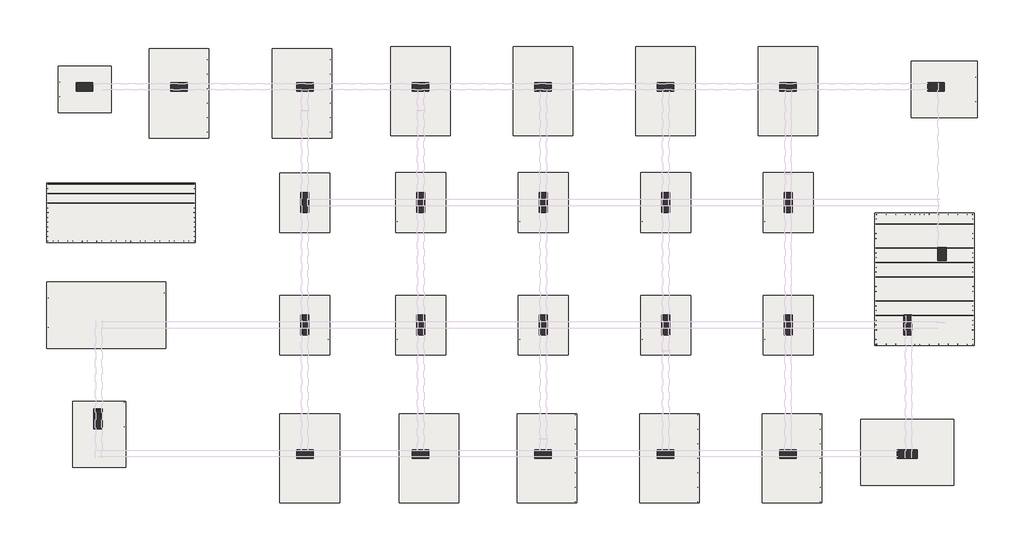
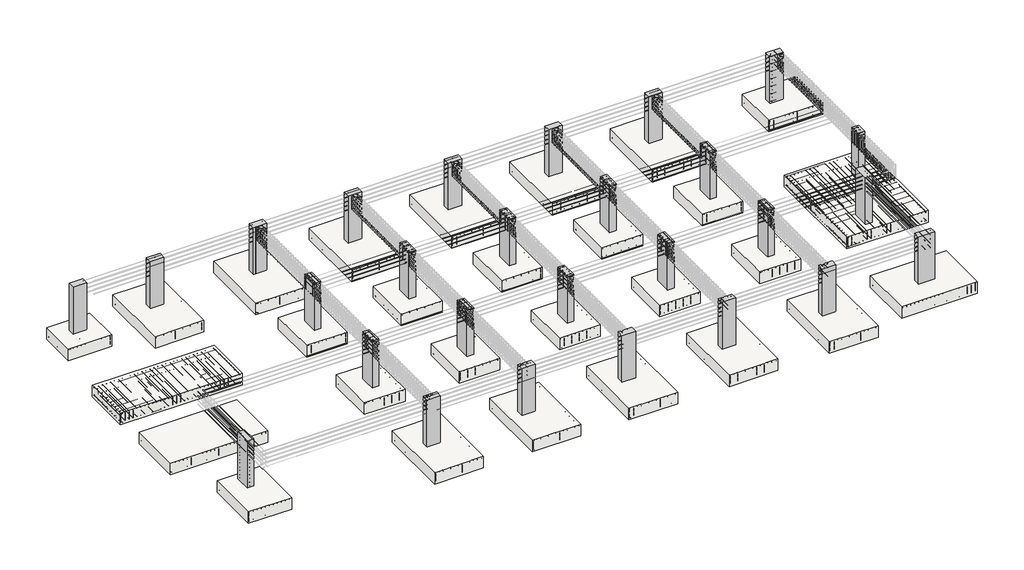
# One storey, part 1 of 16: 28 slabs, 27 columns.
"""IFC4 building model written with IfcOpenShell, lengths in millimetres."""

from ifc_helpers import new_model, si_unit, frame, origin, place, context, project, spatial, polyline, outline, extrude, faceted_brep, transform, mapped, element, save
from components import footing_rectangular_1400x1600x450_119851bf, footing_rectangular_1500x1800x450_b566de6d, footing_rectangular_1600x2000x450_9a9f7728, footing_rectangular_1800x2700x450_79bb3453, footing_rectangular_2000x1700x450_8886efa8, footing_rectangular_2800x2000x450_516ac05f, footing_rectangular_3000x4000x450_ea1acd88, footing_rectangular_3600x2000x450_36af6fae, footing_rectangular_4498x1800x450_c2833046

model = new_model("IFC4")

# Units and contexts
model_context = context("Model", 3, world=origin())
ifc_project = project(units=[si_unit("LENGTHUNIT", "METRE", prefix="MILLI")], contexts=[model_context])

# Site, building, storey
site = spatial("IfcSite", under=ifc_project)
building = spatial("IfcBuilding", under=site)
storey = spatial("IfcBuildingStorey", under=building, Elevation=-1828.8)

# Columns
placement = place(None, origin())
element("IfcColumn", 1, ObjectType="Concrete-Rectangular-Column : 250X400", at=placement, inside=storey, context=model_context, shape_type="SweptSolid", body=[
    extrude(outline(polyline([(10438.1883401, -29.1308992), (10438.1883401, -429.1308992), (10188.1883401, -429.1308992), (10188.1883401, -29.1308992), (10438.1883401, -29.1308992)])), frame((0.0, 0.0, -1828.8), z_axis=(0.0, 0.0, 1.0), x_axis=(1.0, 0.0, 0.0)), (0.0, 0.0, 1.0), 1828.8),
])
element("IfcColumn", 2, ObjectType="Concrete-Rectangular-Column : 250X500", at=placement, inside=storey, context=model_context, shape_type="SweptSolid", body=[
    extrude(outline(polyline([(-15828.3116599, 4945.8691009), (-15328.3116599, 4945.8691009), (-15328.3116599, 4695.8691009), (-15828.3116599, 4695.8691009), (-15828.3116599, 4945.8691009)])), frame((0.0, 0.0, -1828.8), z_axis=(0.0, 0.0, 1.0), x_axis=(1.0, 0.0, 0.0)), (0.0, 0.0, 1.0), 1828.8),
])
element("IfcColumn", 3, ObjectType="Concrete-Rectangular-Column : 250X500", at=placement, inside=storey, context=model_context, shape_type="SweptSolid", body=[
    extrude(outline(polyline([(-12978.3116599, 4945.8691009), (-12478.3116599, 4945.8691009), (-12478.3116599, 4695.8691009), (-12978.3116599, 4695.8691009), (-12978.3116599, 4945.8691009)])), frame((0.0, 0.0, -1828.8), z_axis=(0.0, 0.0, 1.0), x_axis=(1.0, 0.0, 0.0)), (0.0, 0.0, 1.0), 1828.8),
])
element("IfcColumn", 4, ObjectType="Concrete-Rectangular-Column : 250X500", at=placement, inside=storey, context=model_context, shape_type="SweptSolid", body=[
    extrude(outline(polyline([(-9178.2725801, 4945.8691009), (-8678.2725801, 4945.8691009), (-8678.2725801, 4695.8691009), (-9178.2725801, 4695.8691009), (-9178.2725801, 4945.8691009)])), frame((0.0, 0.0, -1828.8), z_axis=(0.0, 0.0, 1.0), x_axis=(1.0, 0.0, 0.0)), (0.0, 0.0, 1.0), 1828.8),
])
element("IfcColumn", 5, ObjectType="Concrete-Rectangular-Column : 250X500", at=placement, inside=storey, context=model_context, shape_type="SweptSolid", body=[
    extrude(outline(polyline([(-5678.2725801, 4945.8691009), (-5178.2725801, 4945.8691009), (-5178.2725801, 4695.8691009), (-5678.2725801, 4695.8691009), (-5678.2725801, 4945.8691009)])), frame((0.0, 0.0, -1828.8), z_axis=(0.0, 0.0, 1.0), x_axis=(1.0, 0.0, 0.0)), (0.0, 0.0, 1.0), 1828.8),
])
element("IfcColumn", 6, ObjectType="Concrete-Rectangular-Column : 250X500", at=placement, inside=storey, context=model_context, shape_type="SweptSolid", body=[
    extrude(outline(polyline([(-1978.2725801, 4945.8691009), (-1478.2725801, 4945.8691009), (-1478.2725801, 4695.8691009), (-1978.2725801, 4695.8691009), (-1978.2725801, 4945.8691009)])), frame((0.0, 0.0, -1828.8), z_axis=(0.0, 0.0, 1.0), x_axis=(1.0, 0.0, 0.0)), (0.0, 0.0, 1.0), 1828.8),
])
element("IfcColumn", 7, ObjectType="Concrete-Rectangular-Column : 250X500", at=placement, inside=storey, context=model_context, shape_type="SweptSolid", body=[
    extrude(outline(polyline([(1721.7274199, 4945.8691009), (2221.7274199, 4945.8691009), (2221.7274199, 4695.8691009), (1721.7274199, 4695.8691009), (1721.7274199, 4945.8691009)])), frame((0.0, 0.0, -1828.8), z_axis=(0.0, 0.0, 1.0), x_axis=(1.0, 0.0, 0.0)), (0.0, 0.0, 1.0), 1828.8),
])
element("IfcColumn", 8, ObjectType="Concrete-Rectangular-Column : 250X500", at=placement, inside=storey, context=model_context, shape_type="SweptSolid", body=[
    extrude(outline(polyline([(5421.7274199, 4945.8691009), (5921.7274199, 4945.8691009), (5921.7274199, 4695.8691009), (5421.7274199, 4695.8691009), (5421.7274199, 4945.8691009)])), frame((0.0, 0.0, -1828.8), z_axis=(0.0, 0.0, 1.0), x_axis=(1.0, 0.0, 0.0)), (0.0, 0.0, 1.0), 1828.8),
])
element("IfcColumn", 9, ObjectType="Concrete-Rectangular-Column : 250X500", at=placement, inside=storey, context=model_context, shape_type="Brep", body=[
    faceted_brep([(9888.1883401, 4942.7630349, 0.0), (9888.1883401, 4692.7630349, 0.0), (10388.1883401, 4692.7630349, 0.0), (10388.1883401, 4942.7630349, 0.0), (9888.1883401, 4942.7630349, -1828.8), (10388.1883401, 4942.7630349, -1828.8), (10388.1883401, 4692.7630349, -1828.8), (9888.1883401, 4692.7630349, -1828.8), (9888.1883401, 4942.7630349, -152.4), (9888.1883401, 4942.7630349, -600.0), (9888.1883401, 4692.7630349, -600.0), (9888.1883401, 4692.7630349, -152.4), (10388.1883401, 4692.7630349, -600.0), (10388.1883401, 4692.7630349, -152.4), (10388.1883401, 4942.7630349, -600.0), (10388.1883401, 4942.7630349, -152.4)], [[[0, 1, 2, 3]], [[4, 5, 6, 7]], [[1, 0, 8, 9, 4, 7, 10, 11]], [[2, 1, 11, 10, 7, 6, 12, 13]], [[3, 2, 13, 12, 6, 5, 14, 15]], [[0, 3, 15, 14, 5, 4, 9, 8]]]),
])
element("IfcColumn", 10, ObjectType="Concrete-Rectangular-Column : 250X500", at=placement, inside=storey, context=model_context, shape_type="SweptSolid", body=[
    extrude(outline(polyline([(5421.7274199, -6154.1308991), (5921.7274199, -6154.1308991), (5921.7274199, -6404.1308991), (5421.7274199, -6404.1308991), (5421.7274199, -6154.1308991)])), frame((0.0, 0.0, -1828.8), z_axis=(0.0, 0.0, 1.0), x_axis=(1.0, 0.0, 0.0)), (0.0, 0.0, 1.0), 1828.8),
])
element("IfcColumn", 11, ObjectType="Concrete-Rectangular-Column : 250X500", at=placement, inside=storey, context=model_context, shape_type="SweptSolid", body=[
    extrude(outline(polyline([(1721.7274199, -6154.1308991), (2221.7274199, -6154.1308991), (2221.7274199, -6404.1308991), (1721.7274199, -6404.1308991), (1721.7274199, -6154.1308991)])), frame((0.0, 0.0, -1828.8), z_axis=(0.0, 0.0, 1.0), x_axis=(1.0, 0.0, 0.0)), (0.0, 0.0, 1.0), 1828.8),
])
element("IfcColumn", 12, ObjectType="Concrete-Rectangular-Column : 250X500", at=placement, inside=storey, context=model_context, shape_type="SweptSolid", body=[
    extrude(outline(polyline([(-1978.2725801, -6154.1308991), (-1478.2725801, -6154.1308991), (-1478.2725801, -6404.1308991), (-1978.2725801, -6404.1308991), (-1978.2725801, -6154.1308991)])), frame((0.0, 0.0, -1828.8), z_axis=(0.0, 0.0, 1.0), x_axis=(1.0, 0.0, 0.0)), (0.0, 0.0, 1.0), 1828.8),
])
element("IfcColumn", 13, ObjectType="Concrete-Rectangular-Column : 250X500", at=placement, inside=storey, context=model_context, shape_type="SweptSolid", body=[
    extrude(outline(polyline([(-5678.2725801, -6154.1308991), (-5178.2725801, -6154.1308991), (-5178.2725801, -6404.1308991), (-5678.2725801, -6404.1308991), (-5678.2725801, -6154.1308991)])), frame((0.0, 0.0, -1828.8), z_axis=(0.0, 0.0, 1.0), x_axis=(1.0, 0.0, 0.0)), (0.0, 0.0, 1.0), 1828.8),
])
element("IfcColumn", 14, ObjectType="Concrete-Rectangular-Column : 250X500", at=placement, inside=storey, context=model_context, shape_type="SweptSolid", body=[
    extrude(outline(polyline([(-9178.2725801, -6154.1308991), (-8678.2725801, -6154.1308991), (-8678.2725801, -6404.1308991), (-9178.2725801, -6404.1308991), (-9178.2725801, -6154.1308991)])), frame((0.0, 0.0, -1828.8), z_axis=(0.0, 0.0, 1.0), x_axis=(1.0, 0.0, 0.0)), (0.0, 0.0, 1.0), 1828.8),
])
element("IfcColumn", 15, ObjectType="Concrete-Rectangular-Column : 250X600", at=placement, inside=storey, context=model_context, shape_type="SweptSolid", body=[
    extrude(outline(polyline([(-8803.2725801, 1620.8691009), (-8803.2725801, 1020.8691009), (-9053.2725801, 1020.8691009), (-9053.2725801, 1620.8691009), (-8803.2725801, 1620.8691009)])), frame((0.0, 0.0, -1828.8), z_axis=(0.0, 0.0, 1.0), x_axis=(1.0, 0.0, 0.0)), (0.0, 0.0, 1.0), 1828.8),
])
element("IfcColumn", 16, ObjectType="Concrete-Rectangular-Column : 250X600", at=placement, inside=storey, context=model_context, shape_type="SweptSolid", body=[
    extrude(outline(polyline([(-5303.2725801, 1622.3111779), (-5303.2725801, 1022.3111779), (-5553.2725801, 1022.3111779), (-5553.2725801, 1622.3111779), (-5303.2725801, 1622.3111779)])), frame((0.0, 0.0, -1828.8), z_axis=(0.0, 0.0, 1.0), x_axis=(1.0, 0.0, 0.0)), (0.0, 0.0, 1.0), 1828.8),
])
element("IfcColumn", 17, ObjectType="Concrete-Rectangular-Column : 250X600", at=placement, inside=storey, context=model_context, shape_type="SweptSolid", body=[
    extrude(outline(polyline([(-1603.2725801, 1622.3111779), (-1603.2725801, 1022.3111779), (-1853.2725801, 1022.3111779), (-1853.2725801, 1622.3111779), (-1603.2725801, 1622.3111779)])), frame((0.0, 0.0, -1828.8), z_axis=(0.0, 0.0, 1.0), x_axis=(1.0, 0.0, 0.0)), (0.0, 0.0, 1.0), 1828.8),
])
element("IfcColumn", 18, ObjectType="Concrete-Rectangular-Column : 250X600", at=placement, inside=storey, context=model_context, shape_type="SweptSolid", body=[
    extrude(outline(polyline([(2096.7274199, 1622.3111779), (2096.7274199, 1022.3111779), (1846.7274199, 1022.3111779), (1846.7274199, 1622.3111779), (2096.7274199, 1622.3111779)])), frame((0.0, 0.0, -1828.8), z_axis=(0.0, 0.0, 1.0), x_axis=(1.0, 0.0, 0.0)), (0.0, 0.0, 1.0), 1828.8),
])
element("IfcColumn", 19, ObjectType="Concrete-Rectangular-Column : 250X600", at=placement, inside=storey, context=model_context, shape_type="SweptSolid", body=[
    extrude(outline(polyline([(5796.7274199, 1622.3111779), (5796.7274199, 1022.3111779), (5546.7274199, 1022.3111779), (5546.7274199, 1622.3111779), (5796.7274199, 1622.3111779)])), frame((0.0, 0.0, -1828.8), z_axis=(0.0, 0.0, 1.0), x_axis=(1.0, 0.0, 0.0)), (0.0, 0.0, 1.0), 1828.8),
])
element("IfcColumn", 20, ObjectType="Concrete-Rectangular-Column : 250X600", at=placement, inside=storey, context=model_context, shape_type="SweptSolid", body=[
    extrude(outline(polyline([(9406.9733834, -2079.1308991), (9406.9733834, -2679.1308991), (9156.9733834, -2679.1308991), (9156.9733834, -2079.1308991), (9406.9733834, -2079.1308991)])), frame((0.0, 0.0, -1828.8), z_axis=(0.0, 0.0, 1.0), x_axis=(1.0, 0.0, 0.0)), (0.0, 0.0, 1.0), 1828.8),
])
element("IfcColumn", 21, ObjectType="Concrete-Rectangular-Column : 250X600", at=placement, inside=storey, context=model_context, shape_type="SweptSolid", body=[
    extrude(outline(polyline([(5796.7274199, -2079.1308991), (5796.7274199, -2679.1308991), (5546.7274199, -2679.1308991), (5546.7274199, -2079.1308991), (5796.7274199, -2079.1308991)])), frame((0.0, 0.0, -1828.8), z_axis=(0.0, 0.0, 1.0), x_axis=(1.0, 0.0, 0.0)), (0.0, 0.0, 1.0), 1828.8),
])
element("IfcColumn", 22, ObjectType="Concrete-Rectangular-Column : 250X600", at=placement, inside=storey, context=model_context, shape_type="SweptSolid", body=[
    extrude(outline(polyline([(2096.7274199, -2079.1308991), (2096.7274199, -2679.1308991), (1846.7274199, -2679.1308991), (1846.7274199, -2079.1308991), (2096.7274199, -2079.1308991)])), frame((0.0, 0.0, -1828.8), z_axis=(0.0, 0.0, 1.0), x_axis=(1.0, 0.0, 0.0)), (0.0, 0.0, 1.0), 1828.8),
])
element("IfcColumn", 23, ObjectType="Concrete-Rectangular-Column : 250X600", at=placement, inside=storey, context=model_context, shape_type="Brep", body=[
    faceted_brep([(-1603.2725801, -2079.1308991, 0.0), (-1853.2725801, -2079.1308991, 0.0), (-1853.2725801, -2679.1308991, 0.0), (-1603.2725801, -2679.1308991, 0.0), (-1603.2725801, -2079.1308991, -1828.8), (-1603.2725801, -2679.1308991, -1828.8), (-1853.2725801, -2679.1308991, -1828.8), (-1853.2725801, -2079.1308991, -1828.8), (-1603.2725801, -2079.1308991, -152.4), (-1603.2725801, -2079.1308991, -600.0), (-1853.2725801, -2079.1308991, -600.0), (-1853.2725801, -2079.1308991, -152.4)], [[[0, 1, 2, 3]], [[4, 5, 6, 7]], [[1, 0, 8, 9, 4, 7, 10, 11]], [[2, 1, 11, 10, 7, 6]], [[3, 2, 6, 5]], [[0, 3, 5, 4, 9, 8]]]),
])
element("IfcColumn", 24, ObjectType="Concrete-Rectangular-Column : 250X600", at=placement, inside=storey, context=model_context, shape_type="SweptSolid", body=[
    extrude(outline(polyline([(-5303.2725801, -2079.1308991), (-5303.2725801, -2679.1308991), (-5553.2725801, -2679.1308991), (-5553.2725801, -2079.1308991), (-5303.2725801, -2079.1308991)])), frame((0.0, 0.0, -1828.8), z_axis=(0.0, 0.0, 1.0), x_axis=(1.0, 0.0, 0.0)), (0.0, 0.0, 1.0), 1828.8),
])
element("IfcColumn", 25, ObjectType="Concrete-Rectangular-Column : 250X600", at=placement, inside=storey, context=model_context, shape_type="Brep", body=[
    faceted_brep([(-8803.2725801, -2079.1308991, 0.0), (-9053.2725801, -2079.1308991, 0.0), (-9053.2725801, -2679.1308991, 0.0), (-8803.2725801, -2679.1308991, 0.0), (-8803.2725801, -2079.1308991, -1828.8), (-8803.2725801, -2679.1308991, -1828.8), (-9053.2725801, -2679.1308991, -1828.8), (-9053.2725801, -2079.1308991, -1828.8), (-8803.2725801, -2079.1308991, -152.4), (-8803.2725801, -2079.1308991, -600.0), (-9053.2725801, -2079.1308991, -600.0), (-9053.2725801, -2079.1308991, -152.4)], [[[0, 1, 2, 3]], [[4, 5, 6, 7]], [[1, 0, 8, 9, 4, 7, 10, 11]], [[2, 1, 11, 10, 7, 6]], [[3, 2, 6, 5]], [[0, 3, 5, 4, 9, 8]]]),
])
element("IfcColumn", 26, ObjectType="Concrete-Rectangular-Column : 250X600", at=placement, inside=storey, context=model_context, shape_type="SweptSolid", body=[
    extrude(outline(polyline([(-15050.5528212, -4909.1308991), (-15050.5528212, -5509.1308991), (-15300.5528212, -5509.1308991), (-15300.5528212, -4909.1308991), (-15050.5528212, -4909.1308991)])), frame((0.0, 0.0, -1828.8), z_axis=(0.0, 0.0, 1.0), x_axis=(1.0, 0.0, 0.0)), (0.0, 0.0, 1.0), 1828.8),
])
element("IfcColumn", 27, ObjectType="Concrete-Rectangular-Column : 250X600", at=placement, inside=storey, context=model_context, shape_type="Brep", body=[
    faceted_brep([(8968.1883401, -6153.1308991, 0.0), (8968.1883401, -6403.1308991, 0.0), (9568.1883401, -6403.1308991, 0.0), (9568.1883401, -6153.1308991, 0.0), (8968.1883401, -6153.1308991, -1828.8), (9568.1883401, -6153.1308991, -1828.8), (9568.1883401, -6403.1308991, -1828.8), (8968.1883401, -6403.1308991, -1828.8), (8968.1883401, -6153.1308991, -152.4), (8968.1883401, -6153.1308991, -600.0), (8968.1883401, -6403.1308991, -600.0), (8968.1883401, -6403.1308991, -152.4)], [[[0, 1, 2, 3]], [[4, 5, 6, 7]], [[1, 0, 8, 9, 4, 7, 10, 11]], [[2, 1, 11, 10, 7, 6]], [[3, 2, 6, 5]], [[0, 3, 5, 4, 9, 8]]]),
])

# Slabs
footing_rectangular_1400x1600x450_shape = footing_rectangular_1400x1600x450_119851bf(model_context)
element("IfcSlab", 28, ObjectType="Footing-Rectangular : 1400X1600X450", at=placement, inside=storey, context=model_context, shape_type="MappedRepresentation", body=[
    mapped(footing_rectangular_1400x1600x450_shape, transform((-15578.3116599, 4745.8691009, -1828.8), x_axis=(0.0, 1.0, 0.0), y_axis=(-1.0, 0.0, 0.0), z_axis=(0.0, 0.0, 1.0))),
])
footing_rectangular_1500x1800x450_shape = footing_rectangular_1500x1800x450_b566de6d(model_context)
element("IfcSlab", 29, ObjectType="Footing-Rectangular : 1500X1800X450", at=placement, inside=storey, context=model_context, shape_type="MappedRepresentation", body=[
    mapped(footing_rectangular_1500x1800x450_shape, transform((-8929.3240997, 1322.3111779, -1828.8), x_axis=(0.0, 1.0, 0.0), y_axis=(-1.0, 0.0, 0.0), z_axis=(0.0, 0.0, 1.0))),
])
element("IfcSlab", 30, ObjectType="Footing-Rectangular : 1500X1800X450", at=placement, inside=storey, context=model_context, shape_type="MappedRepresentation", body=[
    mapped(footing_rectangular_1500x1800x450_shape, transform((-5428.2725801, 1323.7532549, -1828.8), x_axis=(0.0, 1.0, 0.0), y_axis=(-1.0, 0.0, 0.0), z_axis=(0.0, 0.0, 1.0))),
])
element("IfcSlab", 31, ObjectType="Footing-Rectangular : 1500X1800X450", at=placement, inside=storey, context=model_context, shape_type="MappedRepresentation", body=[
    mapped(footing_rectangular_1500x1800x450_shape, transform((-1728.2725801, 1323.7532549, -1828.8), x_axis=(0.0, 1.0, 0.0), y_axis=(-1.0, 0.0, 0.0), z_axis=(0.0, 0.0, 1.0))),
])
element("IfcSlab", 32, ObjectType="Footing-Rectangular : 1500X1800X450", at=placement, inside=storey, context=model_context, shape_type="MappedRepresentation", body=[
    mapped(footing_rectangular_1500x1800x450_shape, transform((1971.7274199, 1323.7532549, -1828.8), x_axis=(0.0, 1.0, 0.0), y_axis=(-1.0, 0.0, 0.0), z_axis=(0.0, 0.0, 1.0))),
])
element("IfcSlab", 33, ObjectType="Footing-Rectangular : 1500X1800X450", at=placement, inside=storey, context=model_context, shape_type="MappedRepresentation", body=[
    mapped(footing_rectangular_1500x1800x450_shape, transform((5671.7274199, 1323.7532549, -1828.8), x_axis=(0.0, 1.0, 0.0), y_axis=(-1.0, 0.0, 0.0), z_axis=(0.0, 0.0, 1.0))),
])
element("IfcSlab", 34, ObjectType="Footing-Rectangular : 1500X1800X450", at=placement, inside=storey, context=model_context, shape_type="MappedRepresentation", body=[
    mapped(footing_rectangular_1500x1800x450_shape, transform((5671.7274199, -2377.6888221, -1828.8), x_axis=(0.0, 1.0, 0.0), y_axis=(-1.0, 0.0, 0.0), z_axis=(0.0, 0.0, 1.0))),
])
element("IfcSlab", 35, ObjectType="Footing-Rectangular : 1500X1800X450", at=placement, inside=storey, context=model_context, shape_type="MappedRepresentation", body=[
    mapped(footing_rectangular_1500x1800x450_shape, transform((1971.7274199, -2377.6888221, -1828.8), x_axis=(0.0, 1.0, 0.0), y_axis=(-1.0, 0.0, 0.0), z_axis=(0.0, 0.0, 1.0))),
])
element("IfcSlab", 36, ObjectType="Footing-Rectangular : 1500X1800X450", at=placement, inside=storey, context=model_context, shape_type="MappedRepresentation", body=[
    mapped(footing_rectangular_1500x1800x450_shape, transform((-1728.2725801, -2377.6888221, -1828.8), x_axis=(0.0, 1.0, 0.0), y_axis=(-1.0, 0.0, 0.0), z_axis=(0.0, 0.0, 1.0))),
])
element("IfcSlab", 37, ObjectType="Footing-Rectangular : 1500X1800X450", at=placement, inside=storey, context=model_context, shape_type="MappedRepresentation", body=[
    mapped(footing_rectangular_1500x1800x450_shape, transform((-5428.2725801, -2377.6888221, -1828.8), x_axis=(0.0, 1.0, 0.0), y_axis=(-1.0, 0.0, 0.0), z_axis=(0.0, 0.0, 1.0))),
])
element("IfcSlab", 38, ObjectType="Footing-Rectangular : 1500X1800X450", at=placement, inside=storey, context=model_context, shape_type="MappedRepresentation", body=[
    mapped(footing_rectangular_1500x1800x450_shape, transform((-8928.2725801, -2377.6888221, -1828.8), x_axis=(0.0, 1.0, 0.0), y_axis=(-1.0, 0.0, 0.0), z_axis=(0.0, 0.0, 1.0))),
])
footing_rectangular_1600x2000x450_shape = footing_rectangular_1600x2000x450_9a9f7728(model_context)
element("IfcSlab", 39, ObjectType="Footing-Rectangular : 1600X2000X450", at=placement, inside=storey, context=model_context, shape_type="MappedRepresentation", body=[
    mapped(footing_rectangular_1600x2000x450_shape, transform((-15130.5528212, -5679.1308991, -1828.8), x_axis=(0.0, 1.0, 0.0), y_axis=(-1.0, 0.0, 0.0), z_axis=(0.0, 0.0, 1.0))),
])
footing_rectangular_1800x2700x450_shape = footing_rectangular_1800x2700x450_79bb3453(model_context)
element("IfcSlab", 40, ObjectType="Footing-Rectangular : 1800X2700X450", at=placement, inside=storey, context=model_context, shape_type="MappedRepresentation", body=[
    mapped(footing_rectangular_1800x2700x450_shape, transform((-12724.5266165, 4620.8691009, -1828.8), x_axis=(0.0, 1.0, 0.0), y_axis=(-1.0, 0.0, 0.0), z_axis=(0.0, 0.0, 1.0))),
])
element("IfcSlab", 41, ObjectType="Footing-Rectangular : 1800X2700X450", at=placement, inside=storey, context=model_context, shape_type="MappedRepresentation", body=[
    mapped(footing_rectangular_1800x2700x450_shape, transform((-9008.0266166, 4620.8691009, -1828.8), x_axis=(0.0, 1.0, 0.0), y_axis=(-1.0, 0.0, 0.0), z_axis=(0.0, 0.0, 1.0))),
])
element("IfcSlab", 42, ObjectType="Footing-Rectangular : 1800X2700X450", at=placement, inside=storey, context=model_context, shape_type="MappedRepresentation", body=[
    mapped(footing_rectangular_1800x2700x450_shape, transform((-5433.0266166, 4692.7630349, -1828.8), x_axis=(0.0, 1.0, 0.0), y_axis=(-1.0, 0.0, 0.0), z_axis=(0.0, 0.0, 1.0))),
])
element("IfcSlab", 43, ObjectType="Footing-Rectangular : 1800X2700X450", at=placement, inside=storey, context=model_context, shape_type="MappedRepresentation", body=[
    mapped(footing_rectangular_1800x2700x450_shape, transform((-1733.0266166, 4692.7630349, -1828.8), x_axis=(0.0, 1.0, 0.0), y_axis=(-1.0, 0.0, 0.0), z_axis=(0.0, 0.0, 1.0))),
])
element("IfcSlab", 44, ObjectType="Footing-Rectangular : 1800X2700X450", at=placement, inside=storey, context=model_context, shape_type="MappedRepresentation", body=[
    mapped(footing_rectangular_1800x2700x450_shape, transform((1966.9733834, 4692.7630349, -1828.8), x_axis=(0.0, 1.0, 0.0), y_axis=(-1.0, 0.0, 0.0), z_axis=(0.0, 0.0, 1.0))),
])
element("IfcSlab", 45, ObjectType="Footing-Rectangular : 1800X2700X450", at=placement, inside=storey, context=model_context, shape_type="MappedRepresentation", body=[
    mapped(footing_rectangular_1800x2700x450_shape, transform((5666.9733834, 4692.7630349, -1828.8), x_axis=(0.0, 1.0, 0.0), y_axis=(-1.0, 0.0, 0.0), z_axis=(0.0, 0.0, 1.0))),
])
element("IfcSlab", 46, ObjectType="Footing-Rectangular : 1800X2700X450", at=placement, inside=storey, context=model_context, shape_type="MappedRepresentation", body=[
    mapped(footing_rectangular_1800x2700x450_shape, transform((5791.9733834, -6408.4085501, -1828.8), x_axis=(0.0, 1.0, 0.0), y_axis=(-1.0, 0.0, 0.0), z_axis=(0.0, 0.0, 1.0))),
])
element("IfcSlab", 47, ObjectType="Footing-Rectangular : 1800X2700X450", at=placement, inside=storey, context=model_context, shape_type="MappedRepresentation", body=[
    mapped(footing_rectangular_1800x2700x450_shape, transform((2091.9733834, -6408.4085501, -1828.8), x_axis=(0.0, 1.0, 0.0), y_axis=(-1.0, 0.0, 0.0), z_axis=(0.0, 0.0, 1.0))),
])
element("IfcSlab", 48, ObjectType="Footing-Rectangular : 1800X2700X450", at=placement, inside=storey, context=model_context, shape_type="MappedRepresentation", body=[
    mapped(footing_rectangular_1800x2700x450_shape, transform((-1608.0266166, -6408.4085501, -1828.8), x_axis=(0.0, 1.0, 0.0), y_axis=(-1.0, 0.0, 0.0), z_axis=(0.0, 0.0, 1.0))),
])
element("IfcSlab", 49, ObjectType="Footing-Rectangular : 1800X2700X450", at=placement, inside=storey, context=model_context, shape_type="MappedRepresentation", body=[
    mapped(footing_rectangular_1800x2700x450_shape, transform((-5178.2725801, -6408.4085501, -1828.8), x_axis=(0.0, 1.0, 0.0), y_axis=(-1.0, 0.0, 0.0), z_axis=(0.0, 0.0, 1.0))),
])
element("IfcSlab", 50, ObjectType="Footing-Rectangular : 1800X2700X450", at=placement, inside=storey, context=model_context, shape_type="MappedRepresentation", body=[
    mapped(footing_rectangular_1800x2700x450_shape, transform((-8778.2725801, -6408.4085501, -1828.8), x_axis=(0.0, 1.0, 0.0), y_axis=(-1.0, 0.0, 0.0), z_axis=(0.0, 0.0, 1.0))),
])
footing_rectangular_2000x1700x450_shape = footing_rectangular_2000x1700x450_8886efa8(model_context)
element("IfcSlab", 51, ObjectType="Footing-Rectangular : 2000X1700X450", at=placement, inside=storey, context=model_context, shape_type="MappedRepresentation", body=[
    mapped(footing_rectangular_2000x1700x450_shape, transform((10388.1883401, 4745.8691009, -1828.8), x_axis=(0.0, 1.0, 0.0), y_axis=(-1.0, 0.0, 0.0), z_axis=(0.0, 0.0, 1.0))),
])
footing_rectangular_2800x2000x450_shape = footing_rectangular_2800x2000x450_516ac05f(model_context)
element("IfcSlab", 52, ObjectType="Footing-Rectangular : 2800X2000X450", at=placement, inside=storey, context=model_context, shape_type="MappedRepresentation", body=[
    mapped(footing_rectangular_2800x2000x450_shape, transform((9268.1883401, -6228.1308991, -1828.8), x_axis=(0.0, 1.0, 0.0), y_axis=(-1.0, 0.0, 0.0), z_axis=(0.0, 0.0, 1.0))),
])
footing_rectangular_3000x4000x450_shape = footing_rectangular_3000x4000x450_ea1acd88(model_context)
element("IfcSlab", 53, ObjectType="Footing-Rectangular : 3000X4000X450", at=placement, inside=storey, context=model_context, shape_type="MappedRepresentation", body=[
    mapped(footing_rectangular_3000x4000x450_shape, transform((9788.1883401, -996.6308991, -1828.8), x_axis=(0.0, 1.0, 0.0), y_axis=(-1.0, 0.0, 0.0), z_axis=(0.0, 0.0, 1.0))),
])
footing_rectangular_3600x2000x450_shape = footing_rectangular_3600x2000x450_36af6fae(model_context)
element("IfcSlab", 54, ObjectType="Footing-Rectangular : 3600X2000X450", at=placement, inside=storey, context=model_context, shape_type="MappedRepresentation", body=[
    mapped(footing_rectangular_3600x2000x450_shape, transform((-14928.3116599, -2079.1308991, -1828.8), x_axis=(0.0, 1.0, 0.0), y_axis=(-1.0, 0.0, 0.0), z_axis=(0.0, 0.0, 1.0))),
])
footing_rectangular_4498x1800x450_shape = footing_rectangular_4498x1800x450_c2833046(model_context)
element("IfcSlab", 55, ObjectType="Footing-Rectangular : 4498X1800X450", at=placement, inside=storey, context=model_context, shape_type="MappedRepresentation", body=[
    mapped(footing_rectangular_4498x1800x450_shape, transform((-14479.278345, 1020.8691009, -1828.8), x_axis=(0.0, 1.0, 0.0), y_axis=(-1.0, 0.0, 0.0), z_axis=(0.0, 0.0, 1.0))),
])

save(model, "model.ifc")

# Revit data of these elements
# Type "Concrete-Rectangular-Column : 250X400"
#   b = 0' - 9.84252"
#   h = 1' - 3.74803"
#   Structural Material [instance default] = Concrete, Cast-in-Place gray
# Type "Concrete-Rectangular-Column : 250X500"
#   b = 0' - 9.84252"
#   h = 1' - 7.68504"
#   Structural Material [instance default] = Concrete, Cast-in-Place gray
# Type "Concrete-Rectangular-Column : 250X600"
#   b = 0' - 9.84252"
#   h = 1' - 11.62205"
#   Structural Material [instance default] = Concrete, Cast-in-Place gray
# Type "Footing-Rectangular : 1400X1600X450"
#   Width = 4' - 7.11811"
#   Length = 5' - 2.99213"
#   Foundation Thickness = 1' - 5.71654"
#   Structural Material [instance default] = Concrete - Cast-in-Place Concrete
#   Assembly Code = ""
# Type "Footing-Rectangular : 1500X1800X450"
#   Width = 5' - 10.86614"
#   Length = 4' - 11.05512"
#   Foundation Thickness = 1' - 5.71654"
#   Structural Material [instance default] = Concrete - Cast-in-Place Concrete
#   Assembly Code = ""
# Type "Footing-Rectangular : 1600X2000X450"
#   Width = 6' - 6.74016"
#   Length = 5' - 2.99213"
#   Foundation Thickness = 1' - 5.71654"
#   Structural Material [instance default] = Concrete - Cast-in-Place Concrete
#   Assembly Code = ""
# Type "Footing-Rectangular : 1800X2700X450"
#   Width = 8' - 10.29921"
#   Length = 5' - 10.86614"
#   Foundation Thickness = 1' - 5.71654"
#   Structural Material [instance default] = Concrete - Cast-in-Place Concrete
#   Assembly Code = ""
# Type "Footing-Rectangular : 2000X1700X450"
#   Width = 5' - 6.92913"
#   Length = 6' - 6.74016"
#   Foundation Thickness = 1' - 5.71654"
#   Structural Material [instance default] = Concrete - Cast-in-Place Concrete
#   Assembly Code = ""
# Type "Footing-Rectangular : 2800X2000X450"
#   Width = 6' - 6.74016"
#   Length = 9' - 2.23622"
#   Foundation Thickness = 1' - 5.71654"
#   Structural Material [instance default] = Concrete - Cast-in-Place Concrete
#   Assembly Code = ""
# Type "Footing-Rectangular : 3000X4000X450"
#   Width = 13' - 1.48031"
#   Length = 9' - 10.11024"
#   Foundation Thickness = 1' - 5.71654"
#   Structural Material [instance default] = Concrete - Cast-in-Place Concrete
#   Assembly Code = ""
# Type "Footing-Rectangular : 3600X2000X450"
#   Width = 6' - 6.74016"
#   Length = 11' - 9.73228"
#   Foundation Thickness = 1' - 5.71654"
#   Structural Material [instance default] = Concrete - Cast-in-Place Concrete
#   Assembly Code = ""
# Type "Footing-Rectangular : 4498X1800X450"
#   Width = 5' - 10.86614"
#   Length = 14' - 9.08661"
#   Foundation Thickness = 1' - 5.71654"
#   Structural Material [instance default] = Concrete - Cast-in-Place Concrete
#   Assembly Code = ""
# Element 1 (IfcColumn, "Concrete-Rectangular-Column : 250X400")
#   Structural Material = Concrete, Cast-in-Place gray
#   Phase Created = New Construction
#   Materials on its faces: "Concrete, Cast-in-Place gray"
# Elements 2, 3, 4, 5, 6, 7, 8, 9, 10, 11, 12, 13, 14 (IfcColumn, "Concrete-Rectangular-Column : 250X500")
#   Structural Material = Concrete, Cast-in-Place gray
#   Phase Created = New Construction
#   Materials on its faces: "Concrete, Cast-in-Place gray"
# Elements 15, 16, 17, 18, 19, 20, 21, 22, 23, 24, 25, 26, 27 (IfcColumn, "Concrete-Rectangular-Column : 250X600")
#   Structural Material = Concrete, Cast-in-Place gray
#   Phase Created = New Construction
#   Materials on its faces: "Concrete, Cast-in-Place gray"
# Element 28 (IfcSlab, "Footing-Rectangular : 1400X1600X450")
#   Structural Material = Concrete - Cast-in-Place Concrete
#   Phase Created = New Construction
#   Materials on its faces: "Concrete - Cast-in-Place Concrete"
# Elements 29, 30, 31, 32, 33, 34, 35, 36, 37, 38 (IfcSlab, "Footing-Rectangular : 1500X1800X450")
#   Structural Material = Concrete - Cast-in-Place Concrete
#   Phase Created = New Construction
#   Materials on its faces: "Concrete - Cast-in-Place Concrete"
# Element 39 (IfcSlab, "Footing-Rectangular : 1600X2000X450")
#   Structural Material = Concrete - Cast-in-Place Concrete
#   Phase Created = New Construction
#   Materials on its faces: "Concrete - Cast-in-Place Concrete"
# Elements 40, 41, 42, 43, 44, 45, 46, 47, 48, 49, 50 (IfcSlab, "Footing-Rectangular : 1800X2700X450")
#   Structural Material = Concrete - Cast-in-Place Concrete
#   Phase Created = New Construction
#   Materials on its faces: "Concrete - Cast-in-Place Concrete"
# Element 51 (IfcSlab, "Footing-Rectangular : 2000X1700X450")
#   Structural Material = Concrete - Cast-in-Place Concrete
#   Phase Created = New Construction
#   Materials on its faces: "Concrete - Cast-in-Place Concrete"
# Element 52 (IfcSlab, "Footing-Rectangular : 2800X2000X450")
#   Structural Material = Concrete - Cast-in-Place Concrete
#   Phase Created = New Construction
#   Materials on its faces: "Concrete - Cast-in-Place Concrete"
# Element 53 (IfcSlab, "Footing-Rectangular : 3000X4000X450")
#   Structural Material = Concrete - Cast-in-Place Concrete
#   Phase Created = New Construction
#   Materials on its faces: "Concrete - Cast-in-Place Concrete"
# Element 54 (IfcSlab, "Footing-Rectangular : 3600X2000X450")
#   Structural Material = Concrete - Cast-in-Place Concrete
#   Phase Created = New Construction
#   Materials on its faces: "Concrete - Cast-in-Place Concrete"
# Element 55 (IfcSlab, "Footing-Rectangular : 4498X1800X450")
#   Structural Material = Concrete - Cast-in-Place Concrete
#   Phase Created = New Construction
#   Materials on its faces: "Concrete - Cast-in-Place Concrete"
# Materials
#   "Concrete, Cast-in-Place gray": class "Concrete", colour RGB 192 192 192, transparency 0, Description = "Cast-in-place concrete", Cost = 0
#   "Concrete - Cast-in-Place Concrete": class "Concrete", colour RGB 192 192 192, transparency 0, Cost = 0
